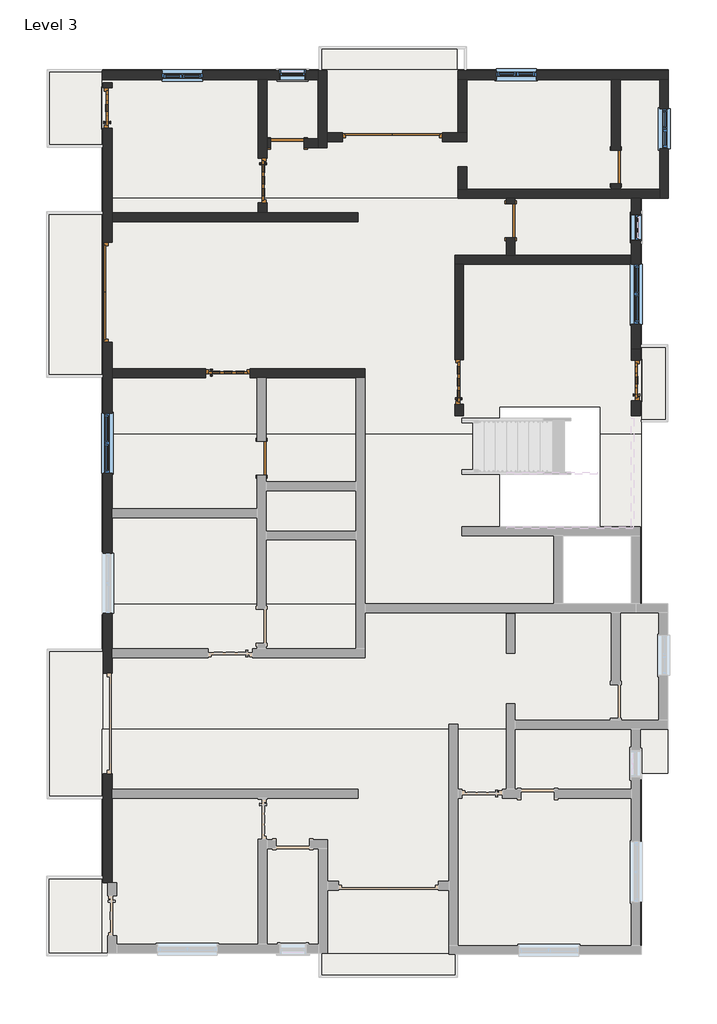
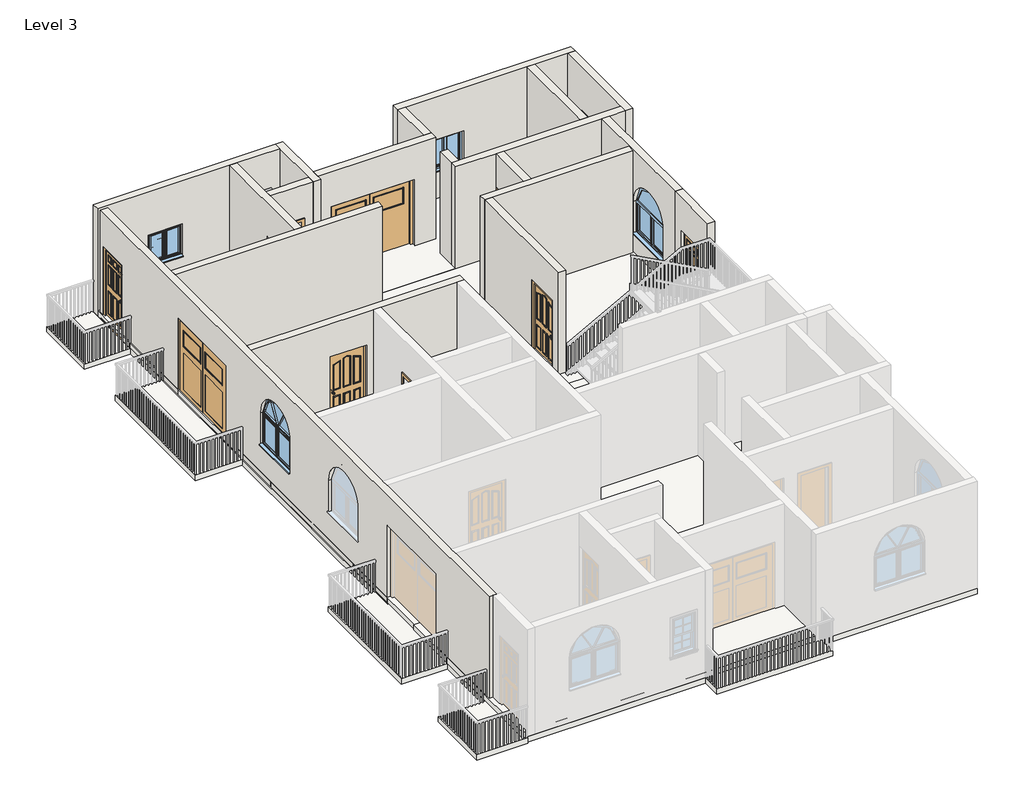
# One storey, part 2 of 7: 19 walls, 11 doors, 10 slabs, 7 windows, 5 roofs.
"""IFC4 building model written with IfcOpenShell, lengths in millimetres."""

from ifc_helpers import new_model, si_unit, point, frame, frame_2d, origin, place, context, project, spatial, polyline, circle_curve, trimmed, segment, composite_curve, outline, extrude, faceted_brep, transform, mapped, element, save
from ifc_brep_helpers import plane_surface, revolved_surface, advanced_brep
from components import doors_extsgl_5_910x2110mm_99758a98, doors_extsgl_5_910x2110mm_d3ca6061, doors_extsgl_6_1010x2110mm_b93c615f, doors_extsgl_6_1010x2110mm_efbaf1af, doors_garage_timber_side_hung_glazing_2270x2050mm_ae99176d, doors_garage_timber_side_hung_glazing_2270x2200mm_badb7014, door_53b1b562, window_679d2811, windows_arched_1360x910mm_c5754810, windows_dbl_w_glazing_bars_910x910mm_41eba874

model = new_model("IFC4")

# Units and contexts
model_context = context("Model", 3, world=origin())
ifc_project = project(units=[si_unit("LENGTHUNIT", "METRE", prefix="MILLI")], contexts=[model_context])

# Site, building, storey
site = spatial("IfcSite", under=ifc_project)
building = spatial("IfcBuilding", under=site)
storey = spatial("IfcBuildingStorey", under=building, Name="Level 3", Elevation=6096.0)

# Doors
placement = place(None, origin())
doors_extsgl_5_910x2110mm_shape = doors_extsgl_5_910x2110mm_99758a98(model_context)
element("IfcDoor", 1, ObjectType="Doors_ExtSgl_5 : 910x2110mm", at=placement, inside=storey, context=model_context, shape_type="MappedRepresentation", body=[
    mapped(doors_extsgl_5_910x2110mm_shape, transform((5761.5890963, 2376.5107951, 6096.0), x_axis=(0.0, 1.0, 0.0), y_axis=(-1.0, 0.0, 0.0), z_axis=(0.0, 0.0, 1.0))),
])
doors_extsgl_5_910x2110mm_2_shape = doors_extsgl_5_910x2110mm_d3ca6061(model_context)
element("IfcDoor", 2, ObjectType="Doors_ExtSgl_5 : 910x2110mm", at=placement, inside=storey, context=model_context, shape_type="MappedRepresentation", body=[
    mapped(doors_extsgl_5_910x2110mm_2_shape, transform((-6229.2013636, 8553.74399, 6096.0), x_axis=(0.0, 1.0, 0.0), y_axis=(-1.0, 0.0, 0.0), z_axis=(0.0, 0.0, 1.0))),
])
doors_extsgl_6_1010x2110mm_shape = doors_extsgl_6_1010x2110mm_b93c615f(model_context)
doors_extsgl_6_1010x2110mm_2_shape = doors_extsgl_6_1010x2110mm_efbaf1af(model_context)
element("IfcDoor", 3, ObjectType="Doors_ExtSgl_6 : 1010x2110mm", at=placement, inside=storey, context=model_context, shape_type="MappedRepresentation", body=[
    mapped(doors_extsgl_6_1010x2110mm_shape, transform((-2709.3109037, 6913.1295584, 6096.0), x_axis=(0.0, -1.0, 0.0), y_axis=(1.0, 0.0, 0.0), z_axis=(0.0, 0.0, 1.0))),
    mapped(doors_extsgl_6_1010x2110mm_2_shape, transform((-2709.3109037, 6913.1295584, 6096.0), x_axis=(0.0, -1.0, 0.0), y_axis=(1.0, 0.0, 0.0), z_axis=(0.0, 0.0, 1.0))),
])
element("IfcDoor", 4, ObjectType="Doors_ExtSgl_6 : 1010x2110mm", at=placement, inside=storey, context=model_context, shape_type="MappedRepresentation", body=[
    mapped(doors_extsgl_6_1010x2110mm_shape, transform((1748.3890963, 2341.0628918, 6096.0), x_axis=(0.0, 1.0, 0.0), y_axis=(-1.0, 0.0, 0.0), z_axis=(0.0, 0.0, 1.0))),
    mapped(doors_extsgl_6_1010x2110mm_2_shape, transform((1748.3890963, 2341.0628918, 6096.0), x_axis=(0.0, 1.0, 0.0), y_axis=(-1.0, 0.0, 0.0), z_axis=(0.0, 0.0, 1.0))),
])
element("IfcDoor", 5, ObjectType="Doors_ExtSgl_6 : 1010x2110mm", at=placement, inside=storey, context=model_context, shape_type="MappedRepresentation", body=[
    mapped(doors_extsgl_6_1010x2110mm_shape, transform((-3496.7442371, 2544.2962251, 6096.0), x_axis=(1.0, 0.0, 0.0), y_axis=(0.0, 1.0, 0.0), z_axis=(0.0, 0.0, 1.0))),
    mapped(doors_extsgl_6_1010x2110mm_2_shape, transform((-3496.7442371, 2544.2962251, 6096.0), x_axis=(1.0, 0.0, 0.0), y_axis=(0.0, 1.0, 0.0), z_axis=(0.0, 0.0, 1.0))),
])
doors_garage_timber_side_hung_glazing_2270x2050mm_shape = doors_garage_timber_side_hung_glazing_2270x2050mm_ae99176d(model_context)
element("IfcDoor", 6, ObjectType="Doors_Garage_Timber_Side_Hung_Glazing : 2270x2050mm", at=placement, inside=storey, context=model_context, shape_type="MappedRepresentation", body=[
    mapped(doors_garage_timber_side_hung_glazing_2270x2050mm_shape, transform((237.0890963, 7890.9962251, 6096.0), x_axis=(1.0, 0.0, 0.0), y_axis=(0.0, 1.0, 0.0), z_axis=(0.0, 0.0, 1.0))),
])
doors_garage_timber_side_hung_glazing_2270x2200mm_shape = doors_garage_timber_side_hung_glazing_2270x2200mm_badb7014(model_context)
element("IfcDoor", 7, ObjectType="Doors_Garage_Timber_Side_Hung_Glazing : 2270x2200mm", at=placement, inside=storey, context=model_context, shape_type="MappedRepresentation", body=[
    mapped(doors_garage_timber_side_hung_glazing_2270x2200mm_shape, transform((-6229.2013636, 4373.0962251, 6096.0), x_axis=(0.0, -1.0, 0.0), y_axis=(1.0, 0.0, 0.0), z_axis=(0.0, 0.0, 1.0))),
])
door_shape = door_53b1b562(model_context)
element("IfcDoor", 8, ObjectType="Single-Flush : 30\" x 80\"", at=placement, inside=storey, context=model_context, shape_type="MappedRepresentation", body=[
    mapped(door_shape, transform((-2150.5109037, 7751.2962251, 6096.0), x_axis=(-1.0, 0.0, 0.0), y_axis=(0.0, -1.0, 0.0), z_axis=(0.0, 0.0, 1.0))),
])
element("IfcDoor", 9, ObjectType="Single-Flush : 30\" x 80\"", at=placement, inside=storey, context=model_context, shape_type="MappedRepresentation", body=[
    mapped(door_shape, transform((2916.7890963, 5998.6962251, 6096.0), x_axis=(0.0, 1.0, 0.0), y_axis=(-1.0, 0.0, 0.0), z_axis=(0.0, 0.0, 1.0))),
])
element("IfcDoor", 10, ObjectType="Single-Flush : 30\" x 80\"", at=placement, inside=storey, context=model_context, shape_type="MappedRepresentation", body=[
    mapped(door_shape, transform((-2734.7109037, 613.8962251, 6096.0), x_axis=(0.0, 1.0, 0.0), y_axis=(-1.0, 0.0, 0.0), z_axis=(0.0, 0.0, 1.0))),
])
element("IfcDoor", 11, ObjectType="Single-Flush : 30\" x 80\"", at=placement, inside=storey, context=model_context, shape_type="MappedRepresentation", body=[
    mapped(door_shape, transform((5304.3890963, 7217.8962251, 6096.0), x_axis=(0.0, 1.0, 0.0), y_axis=(-1.0, 0.0, 0.0), z_axis=(0.0, 0.0, 1.0))),
])

# Roofs
element("IfcRoof", 12, ObjectType="Generic - 12\"", at=placement, inside=storey, context=model_context, shape_type="SweptSolid", body=[
    extrude(outline(polyline([(-6354.2109037, 9427.2527313), (6498.1890963, 9427.2527313), (6498.1890963, 6506.6962251), (-6354.2109037, 6506.6962251), (-6354.2109037, 9427.2527313)])), frame((0.0, 0.0, 6096.0), z_axis=(0.0, 0.0, 1.0), x_axis=(1.0, 0.0, 0.0)), (0.0, 0.0, 1.0), 152.4),
])
element("IfcRoof", 13, ObjectType="Generic - 12\"", at=placement, inside=storey, context=model_context, shape_type="SweptSolid", body=[
    extrude(outline(polyline([(-6330.8013636, -2688.1037749), (6485.4890963, -2688.1037749), (6485.4890963, -6529.1251987), (-6330.8013636, -6529.1251987), (-6330.8013636, -2688.1037749)])), frame((0.0, 0.0, 6096.0), z_axis=(0.0, 0.0, 1.0), x_axis=(1.0, 0.0, 0.0)), (0.0, 0.0, 1.0), 152.4),
])
element("IfcRoof", 14, ObjectType="Generic - 12\"", at=placement, inside=storey, context=model_context, shape_type="SweptSolid", body=[
    extrude(outline(polyline([(-6354.2109037, -5532.9037749), (5863.1890963, -5532.9037749), (5863.1890963, -10612.9037749), (-6354.2109037, -10612.9037749), (-6354.2109037, -5532.9037749)])), frame((0.0, 0.0, 6096.0), z_axis=(0.0, 0.0, 1.0), x_axis=(1.0, 0.0, 0.0)), (0.0, 0.0, 1.0), 152.4),
])
element("IfcRoof", 15, ObjectType="Generic - 12\"", at=placement, inside=storey, context=model_context, shape_type="SweptSolid", body=[
    extrude(outline(polyline([(-6330.8013636, 1160.801054), (-6330.8013636, 6506.6962251), (5875.8890963, 6506.6962251), (5875.8890963, 1160.801054), (4949.8616623, 1160.801054), (4949.8616623, 1784.6684315), (2663.8616623, 1784.6684315), (2663.8616623, 1160.801054), (-6330.8013636, 1160.801054)])), frame((0.0, 0.0, 6096.0), z_axis=(0.0, 0.0, 1.0), x_axis=(1.0, 0.0, 0.0)), (0.0, 0.0, 1.0), 152.4),
])
element("IfcRoof", 16, ObjectType="Generic - 12\"", at=placement, inside=storey, context=model_context, shape_type="SweptSolid", body=[
    extrude(outline(polyline([(-6330.8013636, -2688.1037749), (-6330.8013636, 1160.801054), (2663.8616623, 1160.801054), (2663.8616623, -958.5315685), (4949.8616623, -958.5315685), (4949.8616623, 1160.801054), (5875.8890963, 1160.801054), (5875.8890963, -2688.1037749), (5659.9890963, -2688.1037749), (5659.9890963, -1138.7037749), (4097.8890963, -1138.7037749), (4097.8890963, -2688.1037749), (-6330.8013636, -2688.1037749)])), frame((0.0, 0.0, 6096.0), z_axis=(0.0, 0.0, 1.0), x_axis=(1.0, 0.0, 0.0)), (0.0, 0.0, 1.0), 152.4),
])

# Slabs
element("IfcSlab", 17, ObjectType="Generic - 12\"", at=placement, inside=storey, context=model_context, shape_type="SweptSolid", body=[
    extrude(outline(polyline([(1694.4140963, 9948.3962251), (1694.4140963, -11133.6037749), (-1426.6109037, -11133.6037749), (-1426.6109037, 9948.3962251), (1694.4140963, 9948.3962251)])), frame((0.0, 0.0, 5943.6), z_axis=(0.0, 0.0, 1.0), x_axis=(1.0, 0.0, 0.0)), (0.0, 0.0, 1.0), 152.4),
])
element("IfcSlab", 18, ObjectType="Generic - 12\"", at=placement, inside=storey, context=model_context, shape_type="SweptSolid", body=[
    extrude(outline(polyline([(5875.8890963, 9402.2962251), (5875.8890963, -10638.3037749), (1722.9890963, -10638.3037749), (1722.9890963, 9402.2962251), (5875.8890963, 9402.2962251)]), holes=[polyline([(4949.8616623, 1784.6684315), (2663.8616623, 1784.6684315), (2663.8616623, -958.5315685), (4949.8616623, -958.5315685), (4949.8616623, 1784.6684315)]), polyline([(5659.9890963, -1138.7037749), (4097.8890963, -1138.7037749), (4097.8890963, -2688.1037749), (5659.9890963, -2688.1037749), (5659.9890963, -1138.7037749)])]), frame((0.0, 0.0, 5943.6), z_axis=(0.0, 0.0, 1.0), x_axis=(1.0, 0.0, 0.0)), (0.0, 0.0, 1.0), 152.4),
])
element("IfcSlab", 19, ObjectType="Generic - 12\"", at=placement, inside=storey, context=model_context, shape_type="SweptSolid", body=[
    extrude(outline(polyline([(6498.1890963, 9402.2962251), (6498.1890963, 6506.6962251), (5875.8890963, 6506.6962251), (5875.8890963, 9402.2962251), (6498.1890963, 9402.2962251)])), frame((0.0, 0.0, 5943.6), z_axis=(0.0, 0.0, 1.0), x_axis=(1.0, 0.0, 0.0)), (0.0, 0.0, 1.0), 152.4),
])
element("IfcSlab", 20, ObjectType="Generic - 12\"", at=placement, inside=storey, context=model_context, shape_type="SweptSolid", body=[
    extrude(outline(polyline([(6485.4890963, 3183.81308), (6485.4890963, 1439.3962251), (5863.1890963, 1439.3962251), (5863.1890963, 3183.81308), (6485.4890963, 3183.81308)])), frame((0.0, 0.0, 5943.6), z_axis=(0.0, 0.0, 1.0), x_axis=(1.0, 0.0, 0.0)), (0.0, 0.0, 1.0), 152.4),
])
element("IfcSlab", 21, ObjectType="Generic - 12\"", at=placement, inside=storey, context=model_context, shape_type="SweptSolid", body=[
    extrude(outline(polyline([(6485.4890963, -2688.1037749), (6485.4890963, -5532.9037749), (5863.1890963, -5532.9037749), (5863.1890963, -2688.1037749), (6485.4890963, -2688.1037749)])), frame((0.0, 0.0, 5943.6), z_axis=(0.0, 0.0, 1.0), x_axis=(1.0, 0.0, 0.0)), (0.0, 0.0, 1.0), 152.4),
])
element("IfcSlab", 22, ObjectType="Generic - 12\"", at=placement, inside=storey, context=model_context, shape_type="SweptSolid", body=[
    extrude(outline(polyline([(-6330.8013636, 9427.2527313), (-6330.8013636, 7667.1584215), (-7598.8109037, 7667.1584215), (-7598.8109037, 9427.2527313), (-6330.8013636, 9427.2527313)])), frame((0.0, 0.0, 5943.6), z_axis=(0.0, 0.0, 1.0), x_axis=(1.0, 0.0, 0.0)), (0.0, 0.0, 1.0), 152.4),
])
element("IfcSlab", 23, ObjectType="Generic - 12\"", at=placement, inside=storey, context=model_context, shape_type="SweptSolid", body=[
    extrude(outline(polyline([(-6330.8013636, 6201.8962251), (-6330.8013636, 2455.3962251), (-7614.6859037, 2455.3962251), (-7614.6859037, 6201.8962251), (-6330.8013636, 6201.8962251)])), frame((0.0, 0.0, 5943.6), z_axis=(0.0, 0.0, 1.0), x_axis=(1.0, 0.0, 0.0)), (0.0, 0.0, 1.0), 152.4),
])
element("IfcSlab", 24, ObjectType="Generic - 12\"", at=placement, inside=storey, context=model_context, shape_type="SweptSolid", body=[
    extrude(outline(polyline([(-6330.8013636, -3716.8037749), (-6330.8013636, -7105.2894702), (-7598.8109037, -7105.2894702), (-7598.8109037, -3716.8037749), (-6330.8013636, -3716.8037749)])), frame((0.0, 0.0, 5943.6), z_axis=(0.0, 0.0, 1.0), x_axis=(1.0, 0.0, 0.0)), (0.0, 0.0, 1.0), 152.4),
])
element("IfcSlab", 25, ObjectType="Generic - 12\"", at=placement, inside=storey, context=model_context, shape_type="SweptSolid", body=[
    extrude(outline(polyline([(-6243.0859037, -8868.0845215), (-6243.0859037, -10663.7037749), (-7614.6859037, -10663.7037749), (-7614.6859037, -8868.0845215), (-6243.0859037, -8868.0845215)])), frame((0.0, 0.0, 5943.6), z_axis=(0.0, 0.0, 1.0), x_axis=(1.0, 0.0, 0.0)), (0.0, 0.0, 1.0), 152.4),
])
element("IfcSlab", 26, ObjectType="Generic - 12\"", at=placement, inside=storey, context=model_context, shape_type="SweptSolid", body=[
    extrude(outline(polyline([(-1236.1109037, 9427.2527313), (-1236.1109037, -10612.9037749), (-6354.2109037, -10612.9037749), (-6354.2109037, 9427.2527313), (-1236.1109037, 9427.2527313)])), frame((0.0, 0.0, 5943.6), z_axis=(0.0, 0.0, 1.0), x_axis=(1.0, 0.0, 0.0)), (0.0, 0.0, 1.0), 152.4),
])

# Walls
element("IfcWall", 27, ObjectType="Generic - 9\" w", at=placement, inside=storey, context=model_context, shape_type="Brep", body=[
    faceted_brep([(1722.9890963, 9199.0962251, 6096.0), (1926.1890963, 9199.0962251, 6096.0), (5202.7890963, 9199.0962251, 6096.0), (5405.9890963, 9199.0962251, 6096.0), (6294.9890963, 9199.0962251, 6096.0), (6498.1890963, 9199.0962251, 6096.0), (6498.1890963, 9199.0962251, 9144.0), (6294.9890963, 9199.0962251, 9144.0), (5405.9890963, 9199.0962251, 9144.0), (5202.7890963, 9199.0962251, 9144.0), (1926.1890963, 9199.0962251, 9144.0), (1722.9890963, 9199.0962251, 9144.0), (2588.7890963, 9199.0962251, 7920.4), (3498.7890963, 9199.0962251, 7920.4), (3498.7890963, 9199.0962251, 7010.4), (2588.7890963, 9199.0962251, 7010.4), (1722.9890963, 9402.2962251, 6096.0), (1722.9890963, 9402.2962251, 9144.0), (6498.1890963, 9402.2962251, 9144.0), (6498.1890963, 9402.2962251, 6096.0), (2588.7890963, 9402.2962251, 7920.4), (2588.7890963, 9402.2962251, 7010.4), (3498.7890963, 9402.2962251, 7010.4), (3498.7890963, 9402.2962251, 7920.4)], [[[0, 1, 2, 3, 4, 5, 6, 7, 8, 9, 10, 11], [12, 13, 14, 15]], [[16, 17, 18, 19], [20, 21, 22, 23]], [[5, 4, 3, 2, 1, 0, 16, 19]], [[11, 10, 9, 8, 7, 6, 18, 17]], [[0, 11, 17, 16]], [[6, 5, 19, 18]], [[21, 20, 12, 15]], [[22, 21, 15, 14]], [[23, 22, 14, 13]], [[20, 23, 13, 12]]]),
])
element("IfcWall", 28, ObjectType="Generic - 9\" w", at=placement, inside=storey, context=model_context, shape_type="SweptSolid", body=[
    extrude(outline(polyline([(6506.6962251, 6096.0), (3087.7441284, 6096.0), (3087.7441284, 9144.0), (6506.6962251, 9144.0), (6506.6962251, 6096.0)]), holes=[polyline([(6151.0962251, 8077.2), (5541.4962251, 8077.2), (5541.4962251, 7010.4), (6151.0962251, 7010.4), (6151.0962251, 8077.2)]), composite_curve([segment(polyline([(5016.7786331, 6781.6617803), (5016.7786331, 7691.6617803)]), True, "CONTINUOUS"), segment(trimmed(circle_curve(frame_2d((4336.7786331, 7691.6617803)), 680.0), [point((5016.7786331, 7691.6617803))], [point((3656.7786331, 7691.6617803))], True, "CARTESIAN"), True, "CONTINUOUS"), segment(polyline([(3656.7786331, 7691.6617803), (3656.7786331, 6781.6617803), (5016.7786331, 6781.6617803)]), True, "CONTINUOUS")], self_intersect=False)]), frame((5659.9890963, 0.0, 0.0), z_axis=(1.0, 0.0, 0.0), x_axis=(0.0, 1.0, 0.0)), (0.0, 0.0, 1.0), 203.2),
])
element("IfcWall", 29, ObjectType="Generic - 9\" w", at=placement, inside=storey, context=model_context, shape_type="AdvancedBrep", body=[
    advanced_brep(
    [(-6330.8013636, 3238.0962251, 6096.0), (-6330.8013636, -4267.1251987, 6096.0), (-6330.8013636, -4267.1251987, 8296.0), (-6330.8013636, -6537.1251987, 8296.0), (-6330.8013636, -6537.1251987, 6096.0), (-6330.8013636, -9007.7845215, 6096.0), (-6330.8013636, -9007.7845215, 9144.0), (-6330.8013636, 9129.8816143, 9144.0), (-6330.8013636, 9129.8816143, 6096.0), (-6330.8013636, 9008.7773233, 6096.0), (-6330.8013636, 9008.7773233, 8206.0), (-6330.8013636, 8098.7773233, 8206.0), (-6330.8013636, 8098.7773233, 6096.0), (-6330.8013636, 5508.0962251, 6096.0), (-6330.8013636, 5508.0962251, 8296.0), (-6330.8013636, 3238.0962251, 8296.0), (-6330.8013636, 276.7962251, 7010.4), (-6330.8013636, 1636.7962251, 7010.4), (-6330.8013636, 1636.7962251, 7920.4), (-6330.8013636, 276.7962251, 7920.4), (-6330.8013636, -1538.2037749, 7010.4), (-6330.8013636, -1538.2037749, 7920.4), (-6330.8013636, -2898.2037749, 7920.4), (-6330.8013636, -2898.2037749, 7010.4), (-6127.6013636, -4267.1251987, 8296.0), (-6127.6013636, -4267.1251987, 6096.0), (-6127.6013636, -3907.3037749, 6096.0), (-6127.6013636, -3704.1037749, 6096.0), (-6127.6013636, -732.3037749, 6096.0), (-6127.6013636, -529.1037749, 6096.0), (-6127.6013636, 2442.6962251, 6096.0), (-6127.6013636, 2645.8962251, 6096.0), (-6127.6013636, 3238.0962251, 6096.0), (-6127.6013636, 3238.0962251, 8296.0), (-6127.6013636, 5508.0962251, 8296.0), (-6127.6013636, 5508.0962251, 6096.0), (-6127.6013636, 5973.2962251, 6096.0), (-6127.6013636, 6176.4962251, 6096.0), (-6127.6013636, 8098.7773233, 6096.0), (-6127.6013636, 8098.7773233, 8206.0), (-6127.6013636, 9008.7773233, 8206.0), (-6127.6013636, 9008.7773233, 6096.0), (-6127.6013636, 9129.8816143, 6096.0), (-6127.6013636, 9129.8816143, 9144.0), (-6127.6013636, 6176.4962251, 9144.0), (-6127.6013636, 5973.2962251, 9144.0), (-6127.6013636, 2645.8962251, 9144.0), (-6127.6013636, 2442.6962251, 9144.0), (-6127.6013636, -529.1037749, 9144.0), (-6127.6013636, -732.3037749, 9144.0), (-6127.6013636, -3704.1037749, 9144.0), (-6127.6013636, -3907.3037749, 9144.0), (-6127.6013636, -6896.9466225, 9144.0), (-6127.6013636, -7100.1466225, 9144.0), (-6127.6013636, -9007.7845215, 9144.0), (-6127.6013636, -9007.7845215, 6096.0), (-6127.6013636, -7100.1466225, 6096.0), (-6127.6013636, -6896.9466225, 6096.0), (-6127.6013636, -6537.1251987, 6096.0), (-6127.6013636, -6537.1251987, 8296.0), (-6127.6013636, 276.7962251, 7010.4), (-6127.6013636, 276.7962251, 7920.4), (-6127.6013636, 1636.7962251, 7920.4), (-6127.6013636, 1636.7962251, 7010.4), (-6127.6013636, -1538.2037749, 7010.4), (-6127.6013636, -2898.2037749, 7010.4), (-6127.6013636, -2898.2037749, 7920.4), (-6127.6013636, -1538.2037749, 7920.4), (-6229.2013636, -9007.7845215, 6096.0), (-6229.2013636, -9007.7845215, 9144.0)],
    [
        (0, 1),
        (1, 2),
        (2, 3),
        (3, 4),
        (4, 5),
        (5, 6),
        (6, 7),
        (7, 8),
        (8, 9),
        (9, 10),
        (10, 11),
        (11, 12),
        (12, 13),
        (13, 14),
        (14, 15),
        (15, 0),
        (16, 17),
        (17, 18),
        (18, 19, circle_curve(frame((-6330.8013636, 956.7962251, 7920.4), z_axis=(1.0, 0.0, 0.0), x_axis=(0.0, 1.0, 0.0)), 680.0)),
        (19, 16),
        (20, 21),
        (21, 22, circle_curve(frame((-6330.8013636, -2218.2037749, 7920.4), z_axis=(1.0, 0.0, 0.0), x_axis=(0.0, -1.0, 0.0)), 680.0)),
        (22, 23),
        (23, 20),
        (24, 25),
        (25, 26),
        (26, 27),
        (27, 28),
        (28, 29),
        (29, 30),
        (30, 31),
        (31, 32),
        (32, 33),
        (33, 34),
        (34, 35),
        (35, 36),
        (36, 37),
        (37, 38),
        (38, 39),
        (39, 40),
        (40, 41),
        (41, 42),
        (42, 43),
        (43, 44),
        (44, 45),
        (45, 46),
        (46, 47),
        (47, 48),
        (48, 49),
        (49, 50),
        (50, 51),
        (51, 52),
        (52, 53),
        (53, 54),
        (54, 55),
        (55, 56),
        (56, 57),
        (57, 58),
        (58, 59),
        (59, 24),
        (60, 61),
        (61, 62, circle_curve(frame((-6127.6013636, 956.7962251, 7920.4), z_axis=(-1.0, 0.0, 0.0), x_axis=(0.0, 1.0, 0.0)), 680.0)),
        (62, 63),
        (63, 60),
        (64, 65),
        (65, 66),
        (66, 67, circle_curve(frame((-6127.6013636, -2218.2037749, 7920.4), z_axis=(-1.0, 0.0, 0.0), x_axis=(0.0, -1.0, 0.0)), 680.0)),
        (67, 64),
        (41, 9),
        (8, 42),
        (12, 38),
        (35, 13),
        (55, 68),
        (68, 5),
        (4, 58),
        (25, 1),
        (0, 32),
        (54, 69),
        (69, 6),
        (43, 7),
        (11, 39),
        (40, 10),
        (34, 14),
        (15, 33),
        (3, 59),
        (24, 2),
        (60, 16),
        (19, 61),
        (18, 62),
        (17, 63),
        (20, 64),
        (67, 21),
        (66, 22),
        (65, 23),
    ],
    [
        plane_surface(frame((-6330.8013636, 2442.6962251, 6096.0), z_axis=(-1.0, 0.0, 0.0), x_axis=(0.0, -1.0, 0.0))),
        plane_surface(frame((-6127.6013636, 2442.6962251, 6096.0), z_axis=(1.0, 0.0, 0.0), x_axis=(0.0, 1.0, 0.0))),
        plane_surface(frame((-6330.8013636, 9129.8816143, 6096.0), z_axis=(0.0, 0.0, -1.0), x_axis=(1.0, 0.0, 0.0))),
        plane_surface(frame((-6330.8013636, -9007.7845215, 6096.0), z_axis=(0.0, -1.0, 0.0), x_axis=(1.0, 0.0, 0.0))),
        plane_surface(frame((-6330.8013636, -9007.7845215, 9144.0), z_axis=(0.0, 0.0, 1.0), x_axis=(1.0, 0.0, 0.0))),
        plane_surface(frame((-6330.8013636, 9129.8816143, 9144.0), z_axis=(0.0, 1.0, 0.0), x_axis=(1.0, 0.0, 0.0))),
        plane_surface(frame((-6330.8013636, 8098.7773233, 8206.0), z_axis=(0.0, 1.0, 0.0), x_axis=(1.0, 0.0, 0.0))),
        plane_surface(frame((-6330.8013636, 9008.7773233, 6096.0), z_axis=(0.0, -1.0, 0.0), x_axis=(1.0, 0.0, 0.0))),
        plane_surface(frame((-6330.8013636, 9008.7773233, 8206.0), z_axis=(0.0, 0.0, -1.0), x_axis=(1.0, 0.0, 0.0))),
        plane_surface(frame((-6127.6013636, 5508.0962251, 8296.0), z_axis=(0.0, -1.0, 0.0), x_axis=(-1.0, 0.0, 0.0))),
        plane_surface(frame((-6127.6013636, 3238.0962251, 6096.0), z_axis=(0.0, 1.0, 0.0), x_axis=(-1.0, 0.0, 0.0))),
        plane_surface(frame((-6127.6013636, 3238.0962251, 8296.0), z_axis=(0.0, 0.0, -1.0), x_axis=(-1.0, 0.0, 0.0))),
        plane_surface(frame((-6330.8013636, -6537.1251987, 8296.0), z_axis=(0.0, 1.0, 0.0), x_axis=(1.0, 0.0, 0.0))),
        plane_surface(frame((-6330.8013636, -4267.1251987, 6096.0), z_axis=(0.0, -1.0, 0.0), x_axis=(1.0, 0.0, 0.0))),
        plane_surface(frame((-6330.8013636, -4267.1251987, 8296.0), z_axis=(0.0, 0.0, -1.0), x_axis=(1.0, 0.0, 0.0))),
        plane_surface(frame((-6127.6013636, 276.7962251, 7010.4), z_axis=(0.0, 1.0, 0.0), x_axis=(-1.0, 0.0, 0.0))),
        revolved_surface(polyline([(-6330.8013636, 1636.7962251, 7920.4), (-6127.6013636, 1636.7962251, 7920.4)]), (-6127.6013636, 956.7962251, 7920.4), (-1.0, 0.0, 0.0)),
        plane_surface(frame((-6127.6013636, 1636.7962251, 7920.4), z_axis=(0.0, -1.0, 0.0), x_axis=(-1.0, 0.0, 0.0))),
        plane_surface(frame((-6127.6013636, 1636.7962251, 7010.4), z_axis=(0.0, 0.0, 1.0), x_axis=(-1.0, 0.0, 0.0))),
        plane_surface(frame((-6330.8013636, -1538.2037749, 7010.4), z_axis=(0.0, -1.0, 0.0), x_axis=(1.0, 0.0, 0.0))),
        revolved_surface(polyline([(-6127.6013636, -2898.2037749, 7920.4), (-6330.8013636, -2898.2037749, 7920.4)]), (-6330.8013636, -2218.2037749, 7920.4), (1.0, 0.0, 0.0)),
        plane_surface(frame((-6330.8013636, -2898.2037749, 7920.4), z_axis=(0.0, 1.0, 0.0), x_axis=(1.0, 0.0, 0.0))),
        plane_surface(frame((-6330.8013636, -2898.2037749, 7010.4), z_axis=(0.0, 0.0, 1.0), x_axis=(1.0, 0.0, 0.0))),
    ],
    [
        (0, [[1, 2, 3, 4, 5, 6, 7, 8, 9, 10, 11, 12, 13, 14, 15, 16], [17, 18, 19, 20], [21, 22, 23, 24]]),
        (1, [[25, 26, 27, 28, 29, 30, 31, 32, 33, 34, 35, 36, 37, 38, 39, 40, 41, 42, 43, 44, 45, 46, 47, 48, 49, 50, 51, 52, 53, 54, 55, 56, 57, 58, 59, 60], [61, 62, 63, 64], [65, 66, 67, 68]]),
        (2, [[-42, 69, -9, 70]]),
        (2, [[-13, 71, -38, -37, -36, 72]]),
        (2, [[-58, -57, -56, 73, 74, -5, 75]]),
        (2, [[-32, -31, -30, -29, -28, -27, -26, 76, -1, 77]]),
        (3, [[-6, -74, -73, -55, 78, 79]]),
        (4, [[-7, -79, -78, -54, -53, -52, -51, -50, -49, -48, -47, -46, -45, -44, 80]]),
        (5, [[-8, -80, -43, -70]]),
        (6, [[-12, 81, -39, -71]]),
        (7, [[-10, -69, -41, 82]]),
        (8, [[-11, -82, -40, -81]]),
        (9, [[-35, 83, -14, -72]]),
        (10, [[-33, -77, -16, 84]]),
        (11, [[-34, -84, -15, -83]]),
        (12, [[-4, 85, -59, -75]]),
        (13, [[-2, -76, -25, 86]]),
        (14, [[-3, -86, -60, -85]]),
        (15, [[-61, 87, -20, 88]]),
        (16, [[-62, -88, -19, 89]]),
        (17, [[-63, -89, -18, 90]]),
        (18, [[-64, -90, -17, -87]]),
        (19, [[-21, 91, -68, 92]]),
        (20, [[-22, -92, -67, 93]]),
        (21, [[-23, -93, -66, 94]]),
        (22, [[-24, -94, -65, -91]]),
    ],
),
])
element("IfcWall", 30, ObjectType="Generic - 9\" w", at=placement, inside=storey, context=model_context, shape_type="SweptSolid", body=[
    extrude(outline(polyline([(3087.7441284, 6096.0), (2831.5441284, 6096.0), (2831.5441284, 8206.0), (1921.5441284, 8206.0), (1921.5441284, 6096.0), (1579.0962251, 6096.0), (1579.0962251, 9144.0), (3087.7441284, 9144.0), (3087.7441284, 6096.0)])), frame((5659.9890963, 0.0, 0.0), z_axis=(1.0, 0.0, 0.0), x_axis=(0.0, 1.0, 0.0)), (0.0, 0.0, 1.0), 203.2),
])
element("IfcWall", 31, ObjectType="Generic - 9\" w", at=placement, inside=storey, context=model_context, shape_type="Brep", body=[
    faceted_brep([(-1452.0109037, 9401.8527313, 6096.0), (-6354.2109037, 9401.8527313, 6096.0), (-6354.2109037, 9401.8527313, 9144.0), (-1452.0109037, 9401.8527313, 9144.0), (-4076.7609037, 9401.8527313, 7920.4), (-4986.7609037, 9401.8527313, 7920.4), (-4986.7609037, 9401.8527313, 7010.4), (-4076.7609037, 9401.8527313, 7010.4), (-2334.6609037, 9401.8527313, 8077.2), (-2334.6609037, 9401.8527313, 7010.4), (-1725.0609037, 9401.8527313, 7010.4), (-1725.0609037, 9401.8527313, 8077.2), (-1452.0109037, 9198.6527313, 6096.0), (-1452.0109037, 9198.6527313, 9144.0), (-2607.7109037, 9198.6527313, 9144.0), (-2810.9109037, 9198.6527313, 9144.0), (-6354.2109037, 9198.6527313, 9144.0), (-6354.2109037, 9198.6527313, 6096.0), (-2810.9109037, 9198.6527313, 6096.0), (-2607.7109037, 9198.6527313, 6096.0), (-4076.7609037, 9198.6527313, 7920.4), (-4076.7609037, 9198.6527313, 7010.4), (-4986.7609037, 9198.6527313, 7010.4), (-4986.7609037, 9198.6527313, 7920.4), (-2334.6609037, 9198.6527313, 8077.2), (-1725.0609037, 9198.6527313, 8077.2), (-1725.0609037, 9198.6527313, 7010.4), (-2334.6609037, 9198.6527313, 7010.4)], [[[0, 1, 2, 3], [4, 5, 6, 7], [8, 9, 10, 11]], [[12, 13, 14, 15, 16, 17, 18, 19], [20, 21, 22, 23], [24, 25, 26, 27]], [[1, 0, 12, 19, 18, 17]], [[2, 1, 17, 16]], [[3, 2, 16, 15, 14, 13]], [[0, 3, 13, 12]], [[21, 20, 4, 7]], [[22, 21, 7, 6]], [[23, 22, 6, 5]], [[20, 23, 5, 4]], [[9, 8, 24, 27]], [[10, 9, 27, 26]], [[11, 10, 26, 25]], [[8, 11, 25, 24]]]),
])
element("IfcWall", 32, ObjectType="Generic -4.5\" p", at=placement, inside=storey, context=model_context, shape_type="Brep", body=[
    faceted_brep([(-2810.9109037, 6408.0962251, 8206.0), (-2810.9109037, 6408.0962251, 6096.0), (-2810.9109037, 6176.4962251, 6096.0), (-2810.9109037, 6176.4962251, 9144.0), (-2810.9109037, 9198.6527313, 9144.0), (-2810.9109037, 9198.6527313, 6096.0), (-2810.9109037, 7418.0962251, 6096.0), (-2810.9109037, 7418.0962251, 8206.0), (-2607.7109037, 6176.4962251, 6096.0), (-2607.7109037, 6408.0962251, 6096.0), (-2607.7109037, 6408.0962251, 8206.0), (-2607.7109037, 7418.0962251, 8206.0), (-2607.7109037, 7418.0962251, 6096.0), (-2607.7109037, 7649.6962251, 6096.0), (-2607.7109037, 7852.8962251, 6096.0), (-2607.7109037, 9198.6527313, 6096.0), (-2607.7109037, 9198.6527313, 9144.0), (-2607.7109037, 7852.8962251, 9144.0), (-2607.7109037, 7649.6962251, 9144.0), (-2607.7109037, 6176.4962251, 9144.0)], [[[0, 1, 2, 3, 4, 5, 6, 7]], [[8, 9, 10, 11, 12, 13, 14, 15, 16, 17, 18, 19]], [[6, 5, 15, 14, 13, 12]], [[2, 1, 9, 8]], [[4, 3, 19, 18, 17, 16]], [[3, 2, 8, 19]], [[12, 11, 7, 6]], [[10, 9, 1, 0]], [[11, 10, 0, 7]], [[5, 4, 16, 15]]]),
])
element("IfcWall", 33, ObjectType="Generic -4.5\" p", at=placement, inside=storey, context=model_context, shape_type="Brep", body=[
    faceted_brep([(-6127.6013636, 5973.2962251, 6096.0), (-550.3109037, 5973.2962251, 6096.0), (-550.3109037, 5973.2962251, 9144.0), (-6127.6013636, 5973.2962251, 9144.0), (-6127.6013636, 6176.4962251, 6096.0), (-6127.6013636, 6176.4962251, 9144.0), (-2810.9109037, 6176.4962251, 9144.0), (-2607.7109037, 6176.4962251, 9144.0), (-550.3109037, 6176.4962251, 9144.0), (-550.3109037, 6176.4962251, 6096.0), (-2607.7109037, 6176.4962251, 6096.0), (-2810.9109037, 6176.4962251, 6096.0)], [[[0, 1, 2, 3]], [[4, 5, 6, 7, 8, 9, 10, 11]], [[1, 0, 4, 11, 10, 9]], [[2, 1, 9, 8]], [[3, 2, 8, 7, 6, 5]], [[0, 3, 5, 4]]]),
])
element("IfcWall", 34, ObjectType="Generic -4.5\" p", at=placement, inside=storey, context=model_context, shape_type="Brep", body=[
    faceted_brep([(-1452.0109037, 9401.8527313, 6096.0), (-1452.0109037, 9198.6527313, 6096.0), (-1452.0109037, 7852.8962251, 6096.0), (-1452.0109037, 7649.6962251, 6096.0), (-1452.0109037, 7649.6962251, 9144.0), (-1452.0109037, 7852.8962251, 9144.0), (-1452.0109037, 9198.6527313, 9144.0), (-1452.0109037, 9401.8527313, 9144.0), (-1248.8109037, 9401.8527313, 6096.0), (-1248.8109037, 9401.8527313, 9144.0), (-1248.8109037, 7992.5962251, 9144.0), (-1248.8109037, 7789.3962251, 9144.0), (-1248.8109037, 7649.6962251, 9144.0), (-1248.8109037, 7649.6962251, 6096.0), (-1248.8109037, 7789.3962251, 6096.0), (-1248.8109037, 7992.5962251, 6096.0)], [[[0, 1, 2, 3, 4, 5, 6, 7]], [[8, 9, 10, 11, 12, 13, 14, 15]], [[3, 2, 1, 0, 8, 15, 14, 13]], [[7, 6, 5, 4, 12, 11, 10, 9]], [[4, 3, 13, 12]], [[0, 7, 9, 8]]]),
])
element("IfcWall", 35, ObjectType="Generic -4.5\" p", at=placement, inside=storey, context=model_context, shape_type="SweptSolid", body=[
    extrude(outline(polyline([(6096.0, -2607.7109037), (6096.0, -2531.5109037), (8128.0, -2531.5109037), (8128.0, -1769.5109037), (6096.0, -1769.5109037), (6096.0, -1452.0109037), (9144.0, -1452.0109037), (9144.0, -2607.7109037), (6096.0, -2607.7109037)])), frame((0.0, 7649.6962251, 0.0), z_axis=(0.0, 1.0, 0.0), x_axis=(0.0, 0.0, 1.0)), (0.0, 0.0, 1.0), 203.2),
])
element("IfcWall", 36, ObjectType="Generic -4.5\" p", at=placement, inside=storey, context=model_context, shape_type="Brep", body=[
    faceted_brep([(1372.0890963, 7789.3962251, 8146.0), (1372.0890963, 7789.3962251, 6096.0), (1926.1890963, 7789.3962251, 6096.0), (1926.1890963, 7789.3962251, 9144.0), (-1248.8109037, 7789.3962251, 9144.0), (-1248.8109037, 7789.3962251, 6096.0), (-897.9109037, 7789.3962251, 6096.0), (-897.9109037, 7789.3962251, 8146.0), (1926.1890963, 7992.5962251, 6096.0), (1722.9890963, 7992.5962251, 6096.0), (1372.0890963, 7992.5962251, 6096.0), (1372.0890963, 7992.5962251, 8146.0), (-897.9109037, 7992.5962251, 8146.0), (-897.9109037, 7992.5962251, 6096.0), (-1248.8109037, 7992.5962251, 6096.0), (-1248.8109037, 7992.5962251, 9144.0), (1722.9890963, 7992.5962251, 9144.0), (1926.1890963, 7992.5962251, 9144.0)], [[[0, 1, 2, 3, 4, 5, 6, 7]], [[8, 9, 10, 11, 12, 13, 14, 15, 16, 17]], [[6, 5, 14, 13]], [[2, 1, 10, 9, 8]], [[4, 3, 17, 16, 15]], [[5, 4, 15, 14]], [[3, 2, 8, 17]], [[13, 12, 7, 6]], [[11, 10, 1, 0]], [[12, 11, 0, 7]]]),
])
element("IfcWall", 37, ObjectType="Generic -4.5\" p", at=placement, inside=storey, context=model_context, shape_type="SweptSolid", body=[
    extrude(outline(polyline([(1722.9890963, 7992.5962251), (1722.9890963, 9199.0962251), (1926.1890963, 9199.0962251), (1926.1890963, 7992.5962251), (1722.9890963, 7992.5962251)])), frame((0.0, 0.0, 6096.0), z_axis=(0.0, 0.0, 1.0), x_axis=(1.0, 0.0, 0.0)), (0.0, 0.0, 1.0), 3048.0),
])
element("IfcWall", 38, ObjectType="Generic -4.5\" p", at=placement, inside=storey, context=model_context, shape_type="SweptSolid", body=[
    extrude(outline(polyline([(9199.0962251, 6096.0), (7598.8962251, 6096.0), (7598.8962251, 8128.0), (6836.8962251, 8128.0), (6836.8962251, 6096.0), (6709.8962251, 6096.0), (6709.8962251, 9144.0), (9199.0962251, 9144.0), (9199.0962251, 6096.0)])), frame((5202.7890963, 0.0, 0.0), z_axis=(1.0, 0.0, 0.0), x_axis=(0.0, 1.0, 0.0)), (0.0, 0.0, 1.0), 203.2),
])
element("IfcWall", 39, ObjectType="Generic -4.5\" p", at=placement, inside=storey, context=model_context, shape_type="Brep", body=[
    faceted_brep([(6294.9890963, 9199.0962251, 6096.0), (6294.9890963, 6709.8962251, 6096.0), (6294.9890963, 6506.6962251, 6096.0), (6294.9890963, 6506.6962251, 9144.0), (6294.9890963, 6709.8962251, 9144.0), (6294.9890963, 9199.0962251, 9144.0), (6294.9890963, 8536.4962251, 7920.4), (6294.9890963, 7626.4962251, 7920.4), (6294.9890963, 7626.4962251, 7010.4), (6294.9890963, 8536.4962251, 7010.4), (6498.1890963, 9199.0962251, 6096.0), (6498.1890963, 9199.0962251, 9144.0), (6498.1890963, 6506.6962251, 9144.0), (6498.1890963, 6506.6962251, 6096.0), (6498.1890963, 8536.4962251, 7920.4), (6498.1890963, 8536.4962251, 7010.4), (6498.1890963, 7626.4962251, 7010.4), (6498.1890963, 7626.4962251, 7920.4)], [[[0, 1, 2, 3, 4, 5], [6, 7, 8, 9]], [[10, 11, 12, 13], [14, 15, 16, 17]], [[2, 1, 0, 10, 13]], [[5, 4, 3, 12, 11]], [[3, 2, 13, 12]], [[0, 5, 11, 10]], [[15, 14, 6, 9]], [[16, 15, 9, 8]], [[17, 16, 8, 7]], [[14, 17, 7, 6]]]),
])
element("IfcWall", 40, ObjectType="Generic -4.5\" p", at=placement, inside=storey, context=model_context, shape_type="Brep", body=[
    faceted_brep([(6294.9890963, 6709.8962251, 6096.0), (5405.9890963, 6709.8962251, 6096.0), (5202.7890963, 6709.8962251, 6096.0), (1926.1890963, 6709.8962251, 6096.0), (1722.9890963, 6709.8962251, 6096.0), (1722.9890963, 6709.8962251, 9144.0), (1926.1890963, 6709.8962251, 9144.0), (5202.7890963, 6709.8962251, 9144.0), (5405.9890963, 6709.8962251, 9144.0), (6294.9890963, 6709.8962251, 9144.0), (6294.9890963, 6506.6962251, 6096.0), (6294.9890963, 6506.6962251, 9144.0), (5863.1890963, 6506.6962251, 9144.0), (5659.9890963, 6506.6962251, 9144.0), (3018.3890963, 6506.6962251, 9144.0), (2815.1890963, 6506.6962251, 9144.0), (1722.9890963, 6506.6962251, 9144.0), (1722.9890963, 6506.6962251, 6096.0), (2815.1890963, 6506.6962251, 6096.0), (3018.3890963, 6506.6962251, 6096.0), (5659.9890963, 6506.6962251, 6096.0), (5863.1890963, 6506.6962251, 6096.0)], [[[0, 1, 2, 3, 4, 5, 6, 7, 8, 9]], [[10, 11, 12, 13, 14, 15, 16, 17, 18, 19, 20, 21]], [[4, 3, 2, 1, 0, 10, 21, 20, 19, 18, 17]], [[9, 8, 7, 6, 5, 16, 15, 14, 13, 12, 11]], [[0, 9, 11, 10]], [[5, 4, 17, 16]]]),
])
element("IfcWall", 41, ObjectType="Generic -4.5\" p", at=placement, inside=storey, context=model_context, shape_type="SweptSolid", body=[
    extrude(outline(polyline([(1926.1890963, 7221.6524875), (1926.1890963, 6709.8962251), (1722.9890963, 6709.8962251), (1722.9890963, 7221.6524875), (1926.1890963, 7221.6524875)])), frame((0.0, 0.0, 6096.0), z_axis=(0.0, 0.0, 1.0), x_axis=(1.0, 0.0, 0.0)), (0.0, 0.0, 1.0), 3048.0),
])
element("IfcWall", 42, ObjectType="Generic -4.5\" p", at=placement, inside=storey, context=model_context, shape_type="SweptSolid", body=[
    extrude(outline(polyline([(6506.6962251, 6096.0), (6379.6962251, 6096.0), (6379.6962251, 8128.0), (5617.6962251, 8128.0), (5617.6962251, 6096.0), (5211.2962251, 6096.0), (5211.2962251, 9144.0), (6506.6962251, 9144.0), (6506.6962251, 6096.0)])), frame((2815.1890963, 0.0, 0.0), z_axis=(1.0, 0.0, 0.0), x_axis=(0.0, 1.0, 0.0)), (0.0, 0.0, 1.0), 203.2),
])
element("IfcWall", 43, ObjectType="Generic -4.5\" p", at=placement, inside=storey, context=model_context, shape_type="Brep", body=[
    faceted_brep([(5634.5890963, 5211.2962251, 6096.0), (3018.3890963, 5211.2962251, 6096.0), (2815.1890963, 5211.2962251, 6096.0), (1646.7890963, 5211.2962251, 6096.0), (1646.7890963, 5211.2962251, 9144.0), (2815.1890963, 5211.2962251, 9144.0), (3018.3890963, 5211.2962251, 9144.0), (5634.5890963, 5211.2962251, 9144.0), (5634.5890963, 5008.0962251, 6096.0), (5634.5890963, 5008.0962251, 9144.0), (1849.9890963, 5008.0962251, 9144.0), (1646.7890963, 5008.0962251, 9144.0), (1646.7890963, 5008.0962251, 6096.0), (1849.9890963, 5008.0962251, 6096.0)], [[[0, 1, 2, 3, 4, 5, 6, 7]], [[8, 9, 10, 11, 12, 13]], [[3, 2, 1, 0, 8, 13, 12]], [[7, 6, 5, 4, 11, 10, 9]], [[0, 7, 9, 8]], [[4, 3, 12, 11]]]),
])
element("IfcWall", 44, ObjectType="Generic -4.5\" p", at=placement, inside=storey, context=model_context, shape_type="SweptSolid", body=[
    extrude(outline(polyline([(5008.0962251, 6096.0), (2846.0962251, 6096.0), (2846.0962251, 8206.0), (1836.0962251, 8206.0), (1836.0962251, 6096.0), (1579.0962251, 6096.0), (1579.0962251, 9144.0), (5008.0962251, 9144.0), (5008.0962251, 6096.0)])), frame((1646.7890963, 0.0, 0.0), z_axis=(1.0, 0.0, 0.0), x_axis=(0.0, 1.0, 0.0)), (0.0, 0.0, 1.0), 203.2),
])
element("IfcWall", 45, ObjectType="Generic -4.5\" p", at=placement, inside=storey, context=model_context, shape_type="Brep", body=[
    faceted_brep([(-2991.7109037, 2442.6962251, 8206.0), (-2991.7109037, 2442.6962251, 6096.0), (-2836.3109037, 2442.6962251, 6096.0), (-2633.1109037, 2442.6962251, 6096.0), (-588.4109037, 2442.6962251, 6096.0), (-385.2109037, 2442.6962251, 6096.0), (-385.2109037, 2442.6962251, 9144.0), (-588.4109037, 2442.6962251, 9144.0), (-2633.1109037, 2442.6962251, 9144.0), (-2836.3109037, 2442.6962251, 9144.0), (-6127.6013636, 2442.6962251, 9144.0), (-6127.6013636, 2442.6962251, 6096.0), (-4001.7109037, 2442.6962251, 6096.0), (-4001.7109037, 2442.6962251, 8206.0), (-385.2109037, 2645.8962251, 6096.0), (-2991.7109037, 2645.8962251, 6096.0), (-2991.7109037, 2645.8962251, 8206.0), (-4001.7109037, 2645.8962251, 8206.0), (-4001.7109037, 2645.8962251, 6096.0), (-6127.6013636, 2645.8962251, 6096.0), (-6127.6013636, 2645.8962251, 9144.0), (-385.2109037, 2645.8962251, 9144.0)], [[[0, 1, 2, 3, 4, 5, 6, 7, 8, 9, 10, 11, 12, 13]], [[14, 15, 16, 17, 18, 19, 20, 21]], [[12, 11, 19, 18]], [[5, 4, 3, 2, 1, 15, 14]], [[10, 9, 8, 7, 6, 21, 20]], [[6, 5, 14, 21]], [[18, 17, 13, 12]], [[16, 15, 1, 0]], [[17, 16, 0, 13]], [[11, 10, 20, 19]]]),
])

# Windows
window_shape = window_679d2811(model_context)
element("IfcWindow", 46, ObjectType="Window-Double-Hung : 24\" x 42\"", at=placement, inside=storey, context=model_context, shape_type="MappedRepresentation", body=[
    mapped(window_shape, transform((5761.5890963, 5846.2962251, 6096.0), x_axis=(0.0, -1.0, 0.0), y_axis=(1.0, 0.0, 0.0), z_axis=(0.0, 0.0, 1.0))),
])
element("IfcWindow", 47, ObjectType="Window-Double-Hung : 24\" x 42\"", at=placement, inside=storey, context=model_context, shape_type="MappedRepresentation", body=[
    mapped(window_shape, transform((-2029.8609037, 9300.2527313, 6096.0), x_axis=(1.0, 0.0, 0.0), y_axis=(0.0, 1.0, 0.0), z_axis=(0.0, 0.0, 1.0))),
])
windows_arched_1360x910mm_shape = windows_arched_1360x910mm_c5754810(model_context)
element("IfcWindow", 48, ObjectType="Windows_Arched : 1360x910mm", at=placement, inside=storey, context=model_context, shape_type="MappedRepresentation", body=[
    mapped(windows_arched_1360x910mm_shape, transform((-6220.7447958, 1241.7962251, 5810.4), x_axis=(0.0, 1.0, 0.0), y_axis=(-1.0, 0.0, 0.0), z_axis=(0.0, 0.0, 1.0))),
])
element("IfcWindow", 49, ObjectType="Windows_Arched : 1360x910mm", at=placement, inside=storey, context=model_context, shape_type="MappedRepresentation", body=[
    mapped(windows_arched_1360x910mm_shape, transform((5753.1325284, 4051.7786331, 5581.6617803), x_axis=(0.0, -1.0, 0.0), y_axis=(1.0, 0.0, 0.0), z_axis=(0.0, 0.0, 1.0))),
])
windows_dbl_w_glazing_bars_910x910mm_shape = windows_dbl_w_glazing_bars_910x910mm_41eba874(model_context)
element("IfcWindow", 50, ObjectType="Windows_Dbl_w-Glazing_Bars : 910x910mm", at=placement, inside=storey, context=model_context, shape_type="MappedRepresentation", body=[
    mapped(windows_dbl_w_glazing_bars_910x910mm_shape, transform((6388.1325284, 7951.4962251, 5820.4), x_axis=(0.0, -1.0, 0.0), y_axis=(1.0, 0.0, 0.0), z_axis=(0.0, 0.0, 1.0))),
])
element("IfcWindow", 51, ObjectType="Windows_Dbl_w-Glazing_Bars : 910x910mm", at=placement, inside=storey, context=model_context, shape_type="MappedRepresentation", body=[
    mapped(windows_dbl_w_glazing_bars_910x910mm_shape, transform((3173.7890963, 9292.2396573, 5820.4), x_axis=(1.0, 0.0, 0.0), y_axis=(0.0, 1.0, 0.0), z_axis=(0.0, 0.0, 1.0))),
])
element("IfcWindow", 52, ObjectType="Windows_Dbl_w-Glazing_Bars : 910x910mm", at=placement, inside=storey, context=model_context, shape_type="MappedRepresentation", body=[
    mapped(windows_dbl_w_glazing_bars_910x910mm_shape, transform((-4661.7609037, 9308.7092991, 5820.4), x_axis=(-1.0, 0.0, 0.0), y_axis=(0.0, -1.0, 0.0), z_axis=(0.0, 0.0, 1.0))),
])

save(model, "model.ifc")

# Revit data of these elements
# Type "Doors_ExtSgl_5 : 910x2110mm"
#   Type Mark = "11"
#   Type Comments = "External Single"
#   Operation = "SingleSwingRight"
#   Construction Type Id = "MDOOR"
#   Keynote = "L20"
#   Analytic Construction = "Metal"
#   Wrap Layers (Int) from Ext = 0' - 6.98819"
#   Wrap Layers (Ext) from Ext = 0' - 4.03543"
#   Thickness = 0' - 1.73228"
#   Stile Top of Lock rail = 3' - 3.37008"
#   Stile Top of Frieze Rail = 5' - 4.96063"
#   Stile Top Rail = 0' - 5.90551"
#   Stile Shutting = 0' - 3.14961"
#   Stile Muntin Rail = 0' - 2.95276"
#   Stile Lock Rail = 0' - 6.88976"
#   Stile Intermediate/Frieze = 0' - 3.14961"
#   Stile Hanging = 0' - 3.14961"
#   Stile Bottom Rail = 0' - 6.88976"
#   Rough Width = 2' - 11.82677"
#   Rough Height = 6' - 11.07087"
#   O/A Frame Width = 0' - 2.51969"
#   Heat Transfer Coefficient (U) = 0.651978 BTU/(h·ft²·°F)
#   Handle Z Distance = 3' - 3.37008"
#   Glazing Thickness = 0' - 0.94488"
#   FrameWidth = 0' - 1.65354"
#   FrameOffset - External = 0' - 0.98425"
#   FrameDepth = 0' - 3.50394"
#   Door Panel Width = 2' - 7.77165"
#   Door Panel Thickness = 0' - 1.73228"
#   Door Panel Height = 6' - 6.74016"
#   DONT CHANGE - Panel Width = 0' - 6.52231"
#   Cill Thickness = 0' - 2.14567"
#   Cill Projection = 0' - 1.1811"
#   Handle X Distance = 0' - 2.95276"
#   Height = 6' - 11.07087"
#   Structural Tolerance = 0' - 0.25591"
#   Tolerance = 0' - 0.11811"
#   Undercut = 0' - 0.15748"
#   Width = 2' - 11.82677"
#   Cill Extension = 0' - 0.98425"
#   Cavity Closer Width = 0' - 1.9685"
#   Cavity Closer Offset from Ext = 0' - 4.03543"
#   Cavity Closer Depth = 0' - 3.34646"
#   Vis - Ironmongery = yes
#   Vis - Cavity Closers = yes
#   Define Thermal Properties by = 1
#   Function = 1
#   Material Glass = Door - Glazing
#   Material Door = Door - Panel
#   Material Frame = Door - Frame/Mullion
#   Material Ironmongery = Door - Handle
#   Visual Light Transmittance = 0
#   Solar Heat Gain Coefficient = 0
#   Wall Closure = (empty or 0)
# Type "Doors_ExtSgl_6 : 1010x2110mm"
#   Type Mark = "12"
#   Type Comments = "External Single"
#   Operation = "SingleSwingRight"
#   Construction Type Id = "SGL"
#   Keynote = "L20"
#   Analytic Construction = "Large single-glazed windows"
#   Wrap Layers (Int) from Ext = 0' - 6.98819"
#   Wrap Layers (Ext) from Ext = 0' - 4.03543"
#   Visual Light Transmittance = 0.9
#   Thickness = 0' - 1.73228"
#   Stile Top of Lock rail = 3' - 3.37008"
#   Stile Top Rail = 0' - 5.90551"
#   Stile Shutting = 0' - 3.54331"
#   Stile Muntin Rail = 0' - 3.54331"
#   Stile Lock Rail = 0' - 6.88976"
#   Stile Hanging = 0' - 3.54331"
#   Stile Bottom Rail = 0' - 6.88976"
#   Solar Heat Gain Coefficient = 0.86
#   Rough Width = 3' - 3.76378"
#   Rough Height = 6' - 11.07087"
#   O/A Frame Width = 0' - 2.51969"
#   Heat Transfer Coefficient (U) = 0.979472 BTU/(h·ft²·°F)
#   Handle Z Distance = 3' - 3.37008"
#   Glazing Thickness = 0' - 0.94488"
#   FrameWidth = 0' - 1.65354"
#   FrameOffset - External = 0' - 0.98425"
#   FrameDepth = 0' - 3.50394"
#   Door Panel Width = 2' - 11.70866"
#   Door Panel Thickness = 0' - 1.73228"
#   Door Panel Height = 6' - 6.74016"
#   DONT CHANGE - Panel Width = 0' - 7.17848"
#   Cill Thickness = 0' - 2.14567"
#   Cill Projection = 0' - 1.1811"
#   Handle X Distance = 0' - 2.95276"
#   Height = 6' - 11.07087"
#   Structural Tolerance = 0' - 0.25591"
#   Tolerance = 0' - 0.11811"
#   Undercut = 0' - 0.15748"
#   Width = 3' - 3.76378"
#   Cill Extension = 0' - 0.98425"
#   Cavity Closer Width = 0' - 1.9685"
#   Cavity Closer Offset from Ext = 0' - 4.03543"
#   Cavity Closer Depth = 0' - 3.34646"
#   Vis - Ironmongery = yes
#   Vis - Cavity Closers = yes
#   Define Thermal Properties by = 1
#   Function = 1
#   Material Glass = Door - Glazing
#   Material Door = Door - Panel
#   Material Frame = Door - Frame/Mullion
#   Material Ironmongery = Door - Handle
#   Wall Closure = (empty or 0)
# Type "Doors_Garage_Timber_Side_Hung_Glazing : 2270x2050mm"
#   Type Mark = "8"
#   Type Comments = "External Garage"
#   Operation = "DoubleDoorSingleSwing"
#   Construction Type Id = "GSP4R"
#   Manufacturer = "Revit"
#   Keynote = "L20"
#   Analytic Construction = "1/8 in Pilkington single glazing"
#   Wrap Layers (Ext) from Ext = 0' - 4.03543"
#   Wrap Layers (Int) from Ext = 0' - 6.98819"
#   Visual Light Transmittance = 0.9
#   Thickness = 0' - 1.25984"
#   Stile Top Rail = 0' - 7.87402"
#   Stile Shutting = 0' - 3.93701"
#   Stile Lock Rail = 0' - 7.87402"
#   Stile Hanging = 0' - 6.88976"
#   Stile Bottom Rail = 0' - 9.84252"
#   Solar Heat Gain Coefficient = 0.78
#   Rough Width = 7' - 5.37008"
#   Rough Height = 6' - 8.70866"
#   O/A Frame Width = 0' - 2.51969"
#   Heat Transfer Coefficient (U) = 0.6496 BTU/(h·ft²·°F)
#   Handle Z Distance = 3' - 5.33858"
#   Glazing Panel Height = 1' - 5.71654"
#   FrameWidth = 0' - 1.65354"
#   FrameOffset - External = 0' - 0.98425"
#   FrameDepth = 0' - 3.50394"
#   Door Panel Thickness = 0' - 1.25984"
#   Height = 6' - 8.70866"
#   Structural Tolerance = 0' - 0.31496"
#   Tolerance = 0' - 0.11811"
#   Undercut = 0' - 0.3937"
#   Width = 7' - 5.37008"
#   Cavity Closer Width = 0' - 1.9685"
#   Cavity Closer Offset from Ext = 0' - 4.03543"
#   Cavity Closer Depth = 0' - 3.34646"
#   Vis - Cavity Closers = yes
#   Define Thermal Properties by = 1
#   Function = 1
#   Material Door = Door - Panel
#   Material Frame = Door - Frame/Mullion
#   Material Ironmongery = Door - Handle
#   Wall Closure = (empty or 0)
# Type "Doors_Garage_Timber_Side_Hung_Glazing : 2270x2200mm"
#   Type Mark = "9"
#   Type Comments = "External Garage"
#   Operation = "DoubleDoorSingleSwing"
#   Construction Type Id = "GSP4R"
#   Manufacturer = "Revit"
#   Keynote = "L20"
#   Analytic Construction = "1/8 in Pilkington single glazing"
#   Wrap Layers (Ext) from Ext = 0' - 4.03543"
#   Wrap Layers (Int) from Ext = 0' - 6.98819"
#   Visual Light Transmittance = 0.9
#   Thickness = 0' - 1.25984"
#   Stile Top Rail = 0' - 7.87402"
#   Stile Shutting = 0' - 3.93701"
#   Stile Lock Rail = 0' - 7.87402"
#   Stile Hanging = 0' - 6.88976"
#   Stile Bottom Rail = 0' - 9.84252"
#   Solar Heat Gain Coefficient = 0.78
#   Rough Width = 7' - 5.37008"
#   Rough Height = 7' - 2.61417"
#   O/A Frame Width = 0' - 2.51969"
#   Heat Transfer Coefficient (U) = 0.6496 BTU/(h·ft²·°F)
#   Handle Z Distance = 3' - 5.33858"
#   Glazing Panel Height = 1' - 5.71654"
#   FrameWidth = 0' - 1.65354"
#   FrameOffset - External = 0' - 0.98425"
#   FrameDepth = 0' - 3.50394"
#   Door Panel Thickness = 0' - 1.25984"
#   Height = 7' - 2.61417"
#   Structural Tolerance = 0' - 0.31496"
#   Tolerance = 0' - 0.11811"
#   Undercut = 0' - 0.3937"
#   Width = 7' - 5.37008"
#   Cavity Closer Width = 0' - 1.9685"
#   Cavity Closer Offset from Ext = 0' - 4.03543"
#   Cavity Closer Depth = 0' - 3.34646"
#   Vis - Cavity Closers = yes
#   Define Thermal Properties by = 1
#   Function = 1
#   Material Door = Door - Panel
#   Material Frame = Door - Frame/Mullion
#   Material Ironmongery = Door - Handle
#   Wall Closure = (empty or 0)
# Type "Single-Flush : 30\" x 80\""
#   Type Mark = "5"
#   Construction Type Id = "MDOOR"
#   Assembly Code = "C1020"
#   Analytic Construction = "Metal"
#   Thickness = 0' - 2"
#   Heat Transfer Coefficient (U) = 0.651978 BTU/(h·ft²·°F)
#   Height = 6' - 8"
#   Trim Projection Ext = 0' - 1"
#   Trim Projection Int = 0' - 1"
#   Trim Width = 0' - 3"
#   Width = 2' - 6"
#   Define Thermal Properties by = 1
#   Define Thermal Properties by = 1
#   Door Material = Door - Panel
#   Frame Material = Door - Frame
#   Visual Light Transmittance = 0
#   Solar Heat Gain Coefficient = 0
#   Function = (empty or 0)
#   Wall Closure = (empty or 0)
# Type "Generic - 12\""
#   Assembly Code = "B1020"
#   Layers, outside or top first: 0' - 6" no material (function 1)
# Type "Generic - 12\""
#   Assembly Code = "B1010"
#   Function = 0
#   Layers, outside or top first: 0' - 6" no material (function 1)
# Type "Generic - 9\" w"
#   Assembly Code = "B2010"
#   Layers, outside or top first: 0' - 8" no material (function 1)
# Type "Generic -4.5\" p"
#   Assembly Code = "B2010"
#   Layers, outside or top first: 0' - 8" no material (function 1)
# Type "Window-Double-Hung : 24\" x 42\""
#   Type Mark = "10"
#   Fire Rating = "0.5h"
#   Construction Type Id = "DG-DR"
#   Assembly Code = "B2020100"
#   Analytic Construction = "Double glazing - domestic"
#   Wall Thickness [instance default] = 0' - 6"
#   Window Inset [instance default] = 0' - 0"
#   Visual Light Transmittance = 0.81
#   Thermal Resistance (R) = 1.8146 (h·ft²·°F)/BTU
#   Solar Heat Gain Coefficient = 0.76
#   Muntin Width = 1' - 6"
#   Muntin Height = 1' - 5 1/8"
#   Interior Wall Closure [instance default] = 0' - 1 1/2"
#   Rough Width = 2' - 0 1/2"
#   Rough Height = 3' - 6 1/2"
#   Frame Extension [instance default] = 0' - 1 1/4"
#   Exterior Wall Closure [instance default] = 0' - 0 1/2"
#   Extension Jamb [instance default] = 0' - 1 1/2"
#   Heat Transfer Coefficient (U) = 0.5511 BTU/(h·ft²·°F)
#   Height = 3' - 6"
#   Width = 2' - 0"
#   Define Thermal Properties by = 1
#   Top Muntin Visibility = yes
#   Indicator Visibility [instance default] = yes
#   Extension Jamb Visibility [instance default] = yes
#   Interior Trim Visibility [instance default] = yes
#   Exterior Trim Visibility [instance default] = yes
#   Define Thermal Properties by = 1
#   Bottom Muntin Visibility = yes
#   Muntin Pattern = Muntin Pattern_2x2 : Muntin Pattern_2x2
#   Interior Trim Material = Wood - Stained
#   Interior Trim = Trim-Window-Interior-Flat : Picture Frame
#   Exterior Trim Material = Clad - White
#   Exterior Trim = Trim-Window-Exterior-Flat : with Sill
#   Glass Panel Material = Glass
#   Exterior Frame Material = Clad - White
#   Interior Frame Material = Wood - Stained
#   Wall Closure = (empty or 0)
# Type "Windows_Arched : 1360x910mm"
#   Type Mark = "20"
#   Operation = "UserDefined"
#   Construction Type Id = "GSP4R"
#   Manufacturer = "Revit"
#   Keynote = "L10"
#   Analytic Construction = "1/8 in Pilkington single glazing"
#   Wrap Layers (Ext) from Ext = 0' - 4.03543"
#   Wrap Layers (Int) from Ext = 0' - 6.98819"
#   Window Board Projection = 0' - 0.98425"
#   Window Board Extension = 0' - 0.98425"
#   Visual Light Transmittance = 0.9
#   Solar Heat Gain Coefficient = 0.78
#   Rough Width = 4' - 5.54331"
#   Rough Height = 2' - 11.82677"
#   Height = 2' - 11.82677"
#   Width = 4' - 5.54331"
#   Heat Transfer Coefficient (U) = 0.6496 BTU/(h·ft²·°F)
#   Glazing Thickness = 0' - 0.94488"
#   FrameOffset - External = 0' - 1.9685"
#   Frame Depth = 0' - 2.67717"
#   Default Head Height = 6' - 11.07087"
#   Cill Depth = 0' - 3.44488"
#   Cavity Closer Width = 0' - 1.9685"
#   Cavity Closer Offset from Ext = 0' - 4.03543"
#   Cavity Closer Depth = 0' - 3.34646"
#   Vis - Cavity Closers = yes
#   Define Thermal Properties by = 1
#   Material Trim = Window Frame
#   Material Glass = Glass
#   Material Frame = Window Frame
#   Wall Closure = (empty or 0)
# Type "Windows_Dbl_w-Glazing_Bars : 910x910mm"
#   Type Mark = "33"
#   Operation = "DoublePanelVertical"
#   Construction Type Id = "GSP4R"
#   Manufacturer = "Revit"
#   Keynote = "L10"
#   Analytic Construction = "1/8 in Pilkington single glazing"
#   Wrap Layers (Ext) from Ext = 0' - 4.03543"
#   Wrap Layers (Int) from Ext = 0' - 6.98819"
#   Window Board Projection = 0' - 0.98425"
